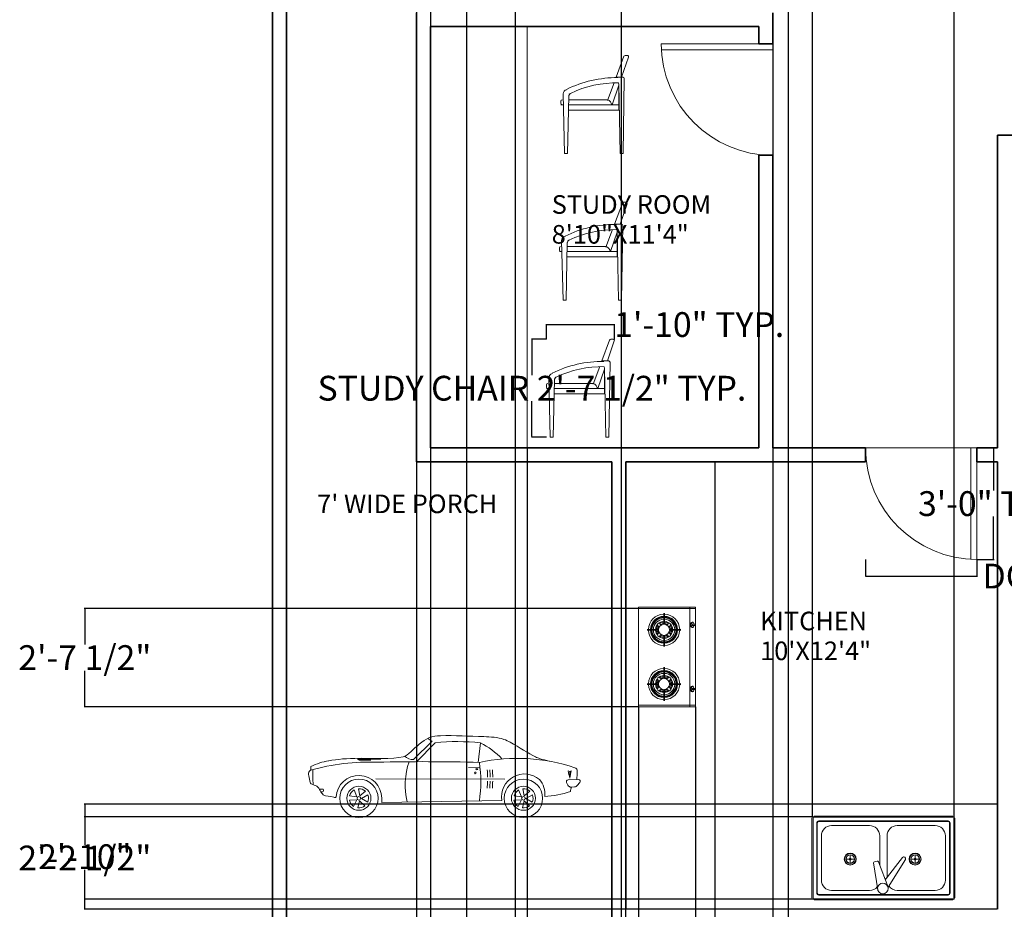
# Model space of a CAD drawing. Units: inches. Extents: x -438 to 102, y -60 to 1091.
# Tile 2 of 20: x -436 to -118, y 205 to 492. Entities that reach past the tile are written whole.
import ezdxf

# ---------------------------------------------------------------- set-up
doc = ezdxf.new("R2010")
doc.units = ezdxf.units.IN
doc.header["$MEASUREMENT"] = 0
for name, color, linetype, lineweight, true_color in [('A-ANNO-DIMS', 217, 'Continuous', 18, 0x93278f), ('A-DOOR', 30, 'Continuous', 18, 0xf26722), ('A-WALL', 2, 'Continuous', 35, 0xf1eb1f), ('C-PROP', 2, 'Continuous', 35, 0xf1eb1f)]:
    doc.layers.add(name, color=color, linetype=linetype, lineweight=lineweight, true_color=true_color)
for name, color, linetype, lineweight in [('A-AREA-IDEN', 4, 'Continuous', 18), ('A-EQPM', 9, 'Continuous', 15), ('A-FLOR-CASE', 7, 'Continuous', 18), ('A-FLOR-FIXT', 9, 'Continuous', 15), ('C-SITE-VEHI', 8, 'Continuous', 15), ('Furniture', 7, 'Continuous', 15)]:
    doc.layers.add(name, color=color, linetype=linetype, lineweight=lineweight)
doc.styles.get("Standard").update_dxf_attribs({"font": 'arial.ttf'})
doc.dimstyles.get("Standard").update_dxf_attribs({"dimtxt": 8, "dimasz": 0.18, "dimexe": 0.18, "dimexo": 0.0625, "dimgap": 0.09, "dimtad": 0, "dimtih": 1, "dimtoh": 1, "dimdec": 4, "dimzin": 0, "dimdsep": 46, "dimlunit": 3, "dimtxsty": 'Standard', "dimcen": 0.09, "dimadec": 0, "dimazin": 0, "dimtfac": 1, "dimtdec": 4, "dimtofl": 0, "dimtmove": 0, "dimatfit": 3, "dimfxl": 1, "dimtolj": 1, "dimtzin": 0, "dimarcsym": 0})

# ---------------------------------------------------------------- blocks, each defined once
blk = doc.blocks.new('*U3')
for p, q in [((72.93, 40.23), (85.8, 53.18)), ((75, 38.82), (88.08, 51.97)), ((119.39, 51.91), (117.92, 38.32)), ((50.13, 41.06), (34.31, 40.98)), ((43.26, 39.85), (35.15, 39.78)), ((35.3, 40.46), (50.13, 40.62)), ((111.09, 34.73), (118.48, 34.64)), ((46.65, 26.83), (136.29, 26.77)), ((179.3, 24.35), (180.25, 22.49)), ((180.37, 26.17), (187.51, 26.41)), ((182.62, 21.14), (184.91, 21.28)), ((186.68, 22.17), (188.51, 24.37)), ((7.45, 19.78), (9.74, 19.8)), ((9.76, 17.93), (8.53, 17.92)), ((10.37, 19.19), (10.38, 18.56)), ((50.87, 13.52), (50.91, 10.52))]:
    blk.add_line(p, q)
for points in [[(35.31, 39.93), (35.3, 40.27, 0.269532), (35.14, 40.54), (34.38, 40.96, 0.575383), (34.15, 40.83), (34.15, 40.49, 0.269532), (34.32, 40.22), (35.08, 39.79, 0.575383)], [(28.49, 15.1), (33.61, 14.4), (31.65, 19.18, 0.199906)], [(34.64, 20.05), (35.56, 14.97), (39.5, 18.31, 0.199906)], [(41.25, 15.74), (36.7, 13.3), (41.09, 10.58, 0.199906)], [(142.85, 15.1), (147.96, 14.4), (146.01, 19.18, 0.199906)], [(148.99, 20.05), (149.91, 14.97), (153.85, 18.31, 0.199906)], [(155.6, 15.74), (151.06, 13.3), (155.45, 10.58, 0.199906)], [(31.31, 7.72), (33.55, 12.37), (28.4, 11.99, 0.199906)], [(39.19, 8.12), (35.46, 11.69), (34.23, 6.67, 0.199906)], [(145.66, 7.72), (147.9, 12.37), (142.75, 11.99, 0.199906)], [(153.54, 8.12), (149.81, 11.69), (148.59, 6.67, 0.199906)]]:
    blk.add_lwpolyline(points, format="xyb", close=True)
for points in [[(181.58, 27.46), (181.53, 31.95), (180.48, 32.43)], [(181.58, 27.46), (181.53, 31.95), (182.57, 32.45)], [(50.91, 10.52), (134.38, 11.83)]]:
    blk.add_lwpolyline(points)
for centre, radius in [((115.89, 31.01), 0.619), ((34.98, 13.35), 13.35), ((34.98, 13.35), 8.35), ((149.33, 13.35), 13.35), ((149.33, 13.35), 8.35), ((34.98, 13.35), 1.25), ((149.33, 13.35), 1.25)]:
    blk.add_circle(centre, radius)
for centre, radius, start, end in [((114.6, 105.09), 59.37, 237.61027, 240.97846), ((103.45, -95), 147.78, 83.81633, 95.97054), ((95.51, 3.91), 53.61, 43.27479, 63.56652), ((73.29, 50.49), 10.26, 230.42401, 268.00854), ((145.17, -84.88), 125.99, 71.52833, 102.12419), ((42.18, -111.35), 149.91, 87.83928, 105.80965), ((20.53, -3.15), 43.06, 98.53035, 116.11198), ((80.1, -1364.13), 1402.96, 88.42296, 91.3179), ((118.31, 22.51), 51.16, 161.43071, 193.23633), ((25.66, 24.94), 94.01, 351.8279, 8.16738), ((184.3, 32.25), 2.49, 357.93203, 71.52833), ((79.16, 30.11), 76.3, 177.57734, 185.52052), ((34.98, 13.35), 15.9, 0.63732, 176.34123), ((45.64, 26.83), 78.76, 0.85201, 4.65562), ((47.43, 26.85), 78.76, 0.85201, 4.65562), ((49.23, 26.87), 78.76, 0.85201, 4.65562), ((150.1, 14.36), 15.92, 49.2263, 189.1528), ((216.26, 37.76), 36.17, 188.46832, 196.53145), ((146.68, 36.98), 36.17, 344.74319, 352.80633), ((116.55, 34.7), 70.29, 353.19423, 357.93203), ((45.64, 26.83), 78.76, 355.26443, 358.86328), ((47.43, 26.85), 78.76, 355.26443, 358.86328), ((49.23, 26.87), 78.76, 355.26443, 358.86328), ((149.4, 16.55), 14.84, 352.72855, 41.66131), ((180.41, 24.92), 1.25, 91.93898, 207.10902), ((182.47, 23.63), 2.49, 207.10902, 273.46767), ((114.25, 37.03), 70.29, 344.3985, 346.93849), ((184.76, 23.76), 2.49, 273.46767, 320.16835), ((187.55, 25.16), 1.25, 320.16835, 91.93898), ((9.75, 19.18), 0.623, 0.63732, 90.63732), ((9.76, 18.55), 0.623, 270.63732, 0.63732), ((162.47, 70.82), 56.18, 271.6865, 290.2774)]:
    blk.add_arc(centre, radius, start, end)
blk.add_ellipse((116.89, 33.59), major_axis=(-0.63, -0.007), ratio=0.610043)
for points, knots in [([(11.39, 38.92), (18.06, 40.19), (30.91, 42.01), (64.77, 40.11), (70.25, 44.91), (82.35, 56.38), (99.18, 57.3), (116.06, 56.35), (133.04, 55.87), (145.24, 49.87), (153.62, 43.8), (161.17, 40.68), (164.92, 39.73), (167.29, 39.15)], [18.629823, 18.629823, 18.629823, 18.629823, 19.527405, 20.700571, 21.107983, 21.608568, 21.92336, 23.151359, 23.716171, 23.908743, 24.77794, 24.943072, 25.187755, 25.187755, 25.187755, 25.187755]), ([(19.11, 14.36), (18.99, 14.21), (18.5, 13.81), (15.35, 15), (9.19, 13.94), (7.26, 22.22), (3.01, 22.66), (1.32, 23.61), (0.64, 26.92), (-0.96, 31.49), (1.54, 32.64), (1.5, 34.06), (1.49, 34.8), (1.49, 35.06), (1.52, 35.3), (1.58, 35.51)], [16.815853, 16.815853, 16.815853, 16.815853, 16.838212, 16.885395, 17.18439, 17.479846, 17.654423, 17.670693, 17.696923, 18.016358, 18.052739, 18.140805, 18.140805, 18.140805, 18.172382, 18.172382, 18.172382, 18.172382])]:
    blk.add_open_spline(points, degree=3, knots=knots)
blk = doc.blocks.new('CHAIR-STUDY')
for p, q in [((9.42, 15.56, -13.5), (6.9, 8.79, -13.5)), ((8.67, 8.79, -13.5), (10.91, 15.29, -13.5)), ((10.54, 15.81, -13.5), (9.79, 15.81, -13.5)), ((6.24, 7.02, -13.5), (4.1, 1.29, -13.5)), ((6.9, 8.79, -13.5), (7.01, 8.79, -13.5)), ((8.16, -15.81, -13.5), (7.76, 6.63, -13.5)), ((7.76, 6.63, -13.5), (7.76, -1.84, -13.5)), ((8.08, 8.79, -13.5), (9.14, 8.79, -13.5)), ((9.14, -15.81, -13.5), (9.54, 8.4, -13.5)), ((-9.76, -15.81, -13.5), (-10.23, 3.39, -13.5)), ((5.6, -0.06, -13.5), (7.76, 6.19, -13.5)), ((-10.94, 0.33, -13.5), (-10.94, 1.12, -13.5)), ((-8.77, -15.81, -13.5), (-8.38, 2.84, -13.5)), ((-8.38, 1.51, -13.5), (4.18, 1.51, -13.5)), ((-10.15, -0.06, -13.5), (-10.94, -0.06, -13.5)), ((-8.38, -0.06, -13.5), (7.76, -0.06, -13.5)), ((7.76, -1.84, -13.5), (-8.38, -1.84, -13.5)), ((7.76, -0.06, -13.5), (5.6, -0.06, -13.5)), ((-8.77, -15.81, -13.5), (-9.76, -15.81, -13.5)), ((9.14, -15.81, -13.5), (8.16, -15.81, -13.5))]:
    blk.add_line(p, q)
for centre, radius, start, end in [((9.79, 15.42, -13.5), 0.394, 90, 159.543), ((10.54, 15.42, -13.5), 0.394, 340.9062, 90), ((7.23, -28.38, -13.5), 37.06, 89.5909, 116.1955), ((7.15, -27.86, -13.5), 34.85, 89.1298, 115.4866), ((7.54, -30.56, -13.5), 39.36, 88.7797, 90.7752), ((7.37, 6.63, -13.5), 0.394, 0, 66.9425), ((9.14, 8.4, -13.5), 0.394, 0, 90), ((-8.76, 3.36, -13.5), 1.47, 106.2385, 178.6251), ((-9.11, 3.69, -13.5), 1.19, 84.4727, 90.6658), ((-7.33, 2.68, -13.5), 1.06, 104.0799, 187.3471), ((7.41, -29.45, -13.5), 36.44, 115.6772, 115.6838), ((-10.54, 1.12, -13.5), 0.394, 90, 180), ((-10.54, 0.33, -13.5), 0.394, 180, 270), ((3.59, -0.28, -13.5), 1.88, 6.4482, 71.4849)]:
    blk.add_arc(centre, radius, start, end)
blk = doc.blocks.new('DOOR-SWING-36')
for p, q in [((-36, 0), (0, 0)), ((-2, 0), (-2, -36)), ((0, 0), (0, -36))]:
    blk.add_line(p, q)
blk.add_arc((0, 0), 36, 180, 270)
blk = doc.blocks.new('*D16')
at = {"layer": 'A-ANNO-DIMS', "color": 0, "lineweight": -2, "transparency": 16777216}
for p, q in [((-265.73, 389.07), (-270.59, 389.07)), ((-270.41, 388.89), (-270.41, 377.48)), ((-270.41, 357.62), (-270.41, 369.03)), ((-265.73, 357.44), (-270.59, 357.44))]:
    blk.add_line(p, q, dxfattribs=at)
at = {"layer": 'A-ANNO-DIMS', "color": 0, "transparency": 16777216}
for points in [[(-270.44, 388.89), (-270.38, 388.89), (-270.41, 389.07)], [(-270.44, 357.62), (-270.38, 357.62), (-270.41, 357.44)]]:
    blk.add_solid(points, dxfattribs=at)
at = {"layer": 'Defpoints', "color": 0, "transparency": 16777216}
for p in [(-270.41, 389.07), (-265.67, 389.07), (-265.67, 357.44)]:
    blk.add_point(p, dxfattribs=at)
at = {"layer": 'A-ANNO-DIMS', "color": 0, "transparency": 16777216, "insert": (-270.41, 373.26), "char_height": 8, "attachment_point": 5}
blk.add_mtext('\\A1;STUDY CHAIR 2\'-7 1/2" TYP.', dxfattribs=at)
blk = doc.blocks.new('*D17')
at = {"layer": 'A-ANNO-DIMS', "color": 0, "lineweight": -2, "transparency": 16777216}
for p, q in [((-265.67, 389.13), (-265.67, 393.99)), ((-265.49, 393.81), (-243.96, 393.81)), ((-243.78, 389.13), (-243.78, 393.99)), ((-243.78, 393.81), (-243.6, 393.81))]:
    blk.add_line(p, q, dxfattribs=at)
at = {"layer": 'A-ANNO-DIMS', "color": 0, "transparency": 16777216}
for points in [[(-265.49, 393.84), (-265.49, 393.78), (-265.67, 393.81)], [(-243.96, 393.84), (-243.96, 393.78), (-243.78, 393.81)]]:
    blk.add_solid(points, dxfattribs=at)
at = {"layer": 'Defpoints', "color": 0, "transparency": 16777216}
for p in [(-243.78, 393.81), (-265.67, 389.07), (-243.78, 389.07)]:
    blk.add_point(p, dxfattribs=at)
at = {"layer": 'A-ANNO-DIMS', "color": 0, "transparency": 16777216, "insert": (-216.4, 393.81), "char_height": 8, "attachment_point": 5}
blk.add_mtext('\\A1;1\'-10" TYP.', dxfattribs=at)
blk = doc.blocks.new('*D20')
at = {"layer": 'A-ANNO-DIMS', "color": 0, "lineweight": -2, "transparency": 16777216}
for p, q in [((-162.74, 317.94), (-162.74, 312.42)), ((-126.74, 317.94), (-126.74, 312.42)), ((-162.56, 312.6), (-126.92, 312.6)), ((-126.74, 312.6), (-126.56, 312.6))]:
    blk.add_line(p, q, dxfattribs=at)
at = {"layer": 'A-ANNO-DIMS', "color": 0, "transparency": 16777216}
for points in [[(-162.56, 312.63), (-162.56, 312.57), (-162.74, 312.6)], [(-126.92, 312.63), (-126.92, 312.57), (-126.74, 312.6)]]:
    blk.add_solid(points, dxfattribs=at)
at = {"layer": 'Defpoints', "color": 0, "transparency": 16777216}
for p in [(-162.74, 318), (-126.74, 318), (-126.74, 312.6)]:
    blk.add_point(p, dxfattribs=at)
at = {"layer": 'A-ANNO-DIMS', "color": 0, "transparency": 16777216, "insert": (-83.97, 312.6), "char_height": 8, "attachment_point": 5}
blk.add_mtext('\\A1;DOOR 3\'-0" TYP.', dxfattribs=at)
blk = doc.blocks.new('*D21')
at = {"layer": 'A-ANNO-DIMS', "color": 0, "lineweight": -2, "transparency": 16777216}
for p, q in [((-126.67, 354), (-121.16, 354)), ((-121.34, 353.82), (-121.34, 340.18)), ((-121.34, 318.18), (-121.34, 331.82)), ((-126.67, 318), (-121.16, 318))]:
    blk.add_line(p, q, dxfattribs=at)
at = {"layer": 'A-ANNO-DIMS', "color": 0, "transparency": 16777216}
for points in [[(-121.37, 353.82), (-121.31, 353.82), (-121.34, 354)], [(-121.37, 318.18), (-121.31, 318.18), (-121.34, 318)]]:
    blk.add_solid(points, dxfattribs=at)
at = {"layer": 'Defpoints', "color": 0, "transparency": 16777216}
for p in [(-126.74, 354), (-121.34, 354), (-126.74, 318)]:
    blk.add_point(p, dxfattribs=at)
at = {"layer": 'A-ANNO-DIMS', "color": 0, "transparency": 16777216, "insert": (-121.34, 336), "char_height": 8, "attachment_point": 5}
blk.add_mtext('\\A1;3\'-0" TYP.', dxfattribs=at)
blk = doc.blocks.new('*D28')
at = {"layer": 'A-ANNO-DIMS', "color": 0, "lineweight": -2, "transparency": 16777216}
for p, q in [((-303.15, 353.94), (-303.15, -48.58)), ((-271.99, 353.94), (-271.99, -48.58)), ((-302.97, -48.4), (-298.36, -48.4)), ((-272.17, -48.4), (-276.78, -48.4))]:
    blk.add_line(p, q, dxfattribs=at)
at = {"layer": 'A-ANNO-DIMS', "color": 0, "transparency": 16777216}
for points in [[(-302.97, -48.37), (-302.97, -48.43), (-303.15, -48.4)], [(-272.17, -48.37), (-272.17, -48.43), (-271.99, -48.4)]]:
    blk.add_solid(points, dxfattribs=at)
at = {"layer": 'Defpoints', "color": 0, "transparency": 16777216}
for p in [(-303.15, 354), (-271.99, 354), (-271.99, -48.4)]:
    blk.add_point(p, dxfattribs=at)
at = {"layer": 'A-ANNO-DIMS', "color": 0, "transparency": 16777216, "insert": (-287.57, -48.4), "char_height": 8, "attachment_point": 5}
blk.add_mtext('\\A1;2\'-7"', dxfattribs=at)
blk = doc.blocks.new('*D29')
at = {"layer": 'A-ANNO-DIMS', "color": 0, "lineweight": -2, "transparency": 16777216}
for p, q in [((-303.15, 494.44), (-303.15, -48.58)), ((-192.65, 494.44), (-192.65, -48.58)), ((-302.97, -48.4), (-267.94, -48.4)), ((-192.83, -48.4), (-227.85, -48.4))]:
    blk.add_line(p, q, dxfattribs=at)
at = {"layer": 'A-ANNO-DIMS', "color": 0, "transparency": 16777216}
for points in [[(-302.97, -48.37), (-302.97, -48.43), (-303.15, -48.4)], [(-192.83, -48.37), (-192.83, -48.43), (-192.65, -48.4)]]:
    blk.add_solid(points, dxfattribs=at)
at = {"layer": 'Defpoints', "color": 0, "transparency": 16777216}
for p in [(-303.15, 494.5), (-192.65, 494.5), (-192.65, -48.4)]:
    blk.add_point(p, dxfattribs=at)
at = {"layer": 'A-ANNO-DIMS', "color": 0, "transparency": 16777216, "insert": (-247.9, -48.4), "char_height": 8, "attachment_point": 5}
blk.add_mtext('\\A1;9\'-2 1/2"', dxfattribs=at)
blk = doc.blocks.new('*D32')
at = {"layer": 'A-ANNO-DIMS', "color": 0, "lineweight": -2, "transparency": 16777216}
for p, q in [((-303.15, 584.44), (-303.15, -48.58)), ((-307.65, 579.94), (-307.65, -48.58)), ((-307.47, -48.4), (-303.33, -48.4)), ((-303.15, -48.4), (-302.97, -48.4))]:
    blk.add_line(p, q, dxfattribs=at)
at = {"layer": 'A-ANNO-DIMS', "color": 0, "transparency": 16777216}
for points in [[(-307.47, -48.37), (-307.47, -48.43), (-307.65, -48.4)], [(-303.33, -48.37), (-303.33, -48.43), (-303.15, -48.4)]]:
    blk.add_solid(points, dxfattribs=at)
at = {"layer": 'Defpoints', "color": 0, "transparency": 16777216}
for p in [(-303.15, 584.5), (-307.65, 580), (-303.15, -48.4)]:
    blk.add_point(p, dxfattribs=at)
at = {"layer": 'A-ANNO-DIMS', "color": 0, "transparency": 16777216, "insert": (-282.92, -48.4), "char_height": 8, "attachment_point": 5}
blk.add_mtext('\\A1;0\'-4 1/2"', dxfattribs=at)
blk = doc.blocks.new('*D33')
at = {"layer": 'A-ANNO-DIMS', "color": 0, "lineweight": -2, "transparency": 16777216}
for p, q in [((-240.15, 349.44), (-240.15, -48.58)), ((-211.32, 349.44), (-211.32, -48.58)), ((-239.97, -48.4), (-236.52, -48.4)), ((-211.5, -48.4), (-214.94, -48.4))]:
    blk.add_line(p, q, dxfattribs=at)
at = {"layer": 'A-ANNO-DIMS', "color": 0, "transparency": 16777216}
for points in [[(-239.97, -48.37), (-239.97, -48.43), (-240.15, -48.4)], [(-211.5, -48.37), (-211.5, -48.43), (-211.32, -48.4)]]:
    blk.add_solid(points, dxfattribs=at)
at = {"layer": 'Defpoints', "color": 0, "transparency": 16777216}
for p in [(-240.15, 349.5), (-211.32, 349.5), (-211.32, -48.4)]:
    blk.add_point(p, dxfattribs=at)
at = {"layer": 'A-ANNO-DIMS', "color": 0, "transparency": 16777216, "insert": (-225.73, -48.4), "char_height": 8, "attachment_point": 5}
blk.add_mtext('\\A1;2\'-5"', dxfattribs=at)
blk = doc.blocks.new('*D34')
at = {"layer": 'A-ANNO-DIMS', "color": 0, "lineweight": -2, "transparency": 16777216}
for p, q in [((-120.21, 238.94), (-414.94, 238.94)), ((-414.76, 238.76), (-414.76, 226.14)), ((-414.76, 205.18), (-414.76, 217.79)), ((-120.21, 205), (-414.94, 205))]:
    blk.add_line(p, q, dxfattribs=at)
at = {"layer": 'A-ANNO-DIMS', "color": 0, "transparency": 16777216}
for points in [[(-414.79, 238.76), (-414.73, 238.76), (-414.76, 238.94)], [(-414.79, 205.18), (-414.73, 205.18), (-414.76, 205)]]:
    blk.add_solid(points, dxfattribs=at)
at = {"layer": 'Defpoints', "color": 0, "transparency": 16777216}
for p in [(-120.15, 238.94), (-414.76, 205), (-120.15, 205)]:
    blk.add_point(p, dxfattribs=at)
at = {"layer": 'A-ANNO-DIMS', "color": 0, "transparency": 16777216, "insert": (-414.76, 221.97), "char_height": 8, "attachment_point": 5}
blk.add_mtext('\\A1;2\'-10"', dxfattribs=at)
blk = doc.blocks.new('*D37')
at = {"layer": 'A-ANNO-DIMS', "color": 0, "lineweight": -2, "transparency": 16777216}
for p, q in [((-179.8, 234.94), (-179.8, 1079.58)), ((-179.62, 1079.4), (-176.98, 1079.4)), ((-134.26, 1079.4), (-136.9, 1079.4)), ((-134.08, 234.94), (-134.08, 1079.58))]:
    blk.add_line(p, q, dxfattribs=at)
at = {"layer": 'A-ANNO-DIMS', "color": 0, "transparency": 16777216}
for points in [[(-179.62, 1079.43), (-179.62, 1079.37), (-179.8, 1079.4)], [(-134.26, 1079.43), (-134.26, 1079.37), (-134.08, 1079.4)]]:
    blk.add_solid(points, dxfattribs=at)
at = {"layer": 'Defpoints', "color": 0, "transparency": 16777216}
for p in [(-134.08, 1079.4), (-179.8, 234.88), (-134.08, 234.88)]:
    blk.add_point(p, dxfattribs=at)
at = {"layer": 'A-ANNO-DIMS', "color": 0, "transparency": 16777216, "insert": (-156.94, 1079.4), "char_height": 8, "attachment_point": 5}
blk.add_mtext('\\A1;3\'-9 1/2"', dxfattribs=at)
blk = doc.blocks.new('*D38')
at = {"layer": 'A-ANNO-DIMS', "color": 0, "lineweight": -2, "transparency": 16777216}
for p, q in [((-179.86, 234.88), (-414.94, 234.88)), ((-414.76, 234.7), (-414.76, 225.8)), ((-414.76, 208.44), (-414.76, 217.34)), ((-179.86, 208.26), (-414.94, 208.26))]:
    blk.add_line(p, q, dxfattribs=at)
at = {"layer": 'A-ANNO-DIMS', "color": 0, "transparency": 16777216}
for points in [[(-414.79, 234.7), (-414.73, 234.7), (-414.76, 234.88)], [(-414.79, 208.44), (-414.73, 208.44), (-414.76, 208.26)]]:
    blk.add_solid(points, dxfattribs=at)
at = {"layer": 'Defpoints', "color": 0, "transparency": 16777216}
for p in [(-414.76, 234.88), (-179.8, 234.88), (-179.8, 208.26)]:
    blk.add_point(p, dxfattribs=at)
at = {"layer": 'A-ANNO-DIMS', "color": 0, "transparency": 16777216, "insert": (-414.76, 221.57), "char_height": 8, "attachment_point": 5}
blk.add_mtext('\\A1;2\'-2 1/2"', dxfattribs=at)
blk = doc.blocks.new('*D39')
at = {"layer": 'A-ANNO-DIMS', "color": 0, "lineweight": -2, "transparency": 16777216}
for p, q in [((-236.04, 302.11), (-414.94, 302.11)), ((-414.76, 301.93), (-414.76, 290.49)), ((-414.76, 270.6), (-414.76, 282.04)), ((-236.04, 270.42), (-414.94, 270.42))]:
    blk.add_line(p, q, dxfattribs=at)
at = {"layer": 'A-ANNO-DIMS', "color": 0, "transparency": 16777216}
for points in [[(-414.79, 301.93), (-414.73, 301.93), (-414.76, 302.11)], [(-414.79, 270.6), (-414.73, 270.6), (-414.76, 270.42)]]:
    blk.add_solid(points, dxfattribs=at)
at = {"layer": 'Defpoints', "color": 0, "transparency": 16777216}
for p in [(-235.98, 302.11), (-414.76, 270.42), (-235.98, 270.42)]:
    blk.add_point(p, dxfattribs=at)
at = {"layer": 'A-ANNO-DIMS', "color": 0, "transparency": 16777216, "insert": (-414.76, 286.27), "char_height": 8, "attachment_point": 5}
blk.add_mtext('\\A1;2\'-7 1/2"', dxfattribs=at)
blk = doc.blocks.new('*D40')
at = {"layer": 'A-ANNO-DIMS', "color": 0, "lineweight": -2, "transparency": 16777216}
for p, q in [((-235.98, 270.35), (-235.98, -48.58)), ((-217.6, 270.35), (-217.6, -48.58)), ((-235.8, -48.4), (-217.78, -48.4)), ((-217.6, -48.4), (-217.42, -48.4))]:
    blk.add_line(p, q, dxfattribs=at)
at = {"layer": 'A-ANNO-DIMS', "color": 0, "transparency": 16777216}
for points in [[(-235.8, -48.37), (-235.8, -48.43), (-235.98, -48.4)], [(-217.78, -48.37), (-217.78, -48.43), (-217.6, -48.4)]]:
    blk.add_solid(points, dxfattribs=at)
at = {"layer": 'Defpoints', "color": 0, "transparency": 16777216}
for p in [(-235.98, 270.42), (-217.6, 270.42), (-217.6, -48.4)]:
    blk.add_point(p, dxfattribs=at)
at = {"layer": 'A-ANNO-DIMS', "color": 0, "transparency": 16777216, "insert": (-197.75, -48.4), "char_height": 8, "attachment_point": 5}
blk.add_mtext('\\A1;1\'-6 1/2"', dxfattribs=at)
blk = doc.blocks.new('*D51')
at = {"layer": 'A-ANNO-DIMS', "color": 0, "lineweight": -2, "transparency": 16777216}
for p, q in [((-291.54, 847), (-291.54, -48.58)), ((-275.79, 847), (-275.79, -48.58)), ((-291.36, -48.4), (-275.97, -48.4)), ((-275.79, -48.4), (-275.61, -48.4))]:
    blk.add_line(p, q, dxfattribs=at)
at = {"layer": 'A-ANNO-DIMS', "color": 0, "transparency": 16777216}
for points in [[(-291.36, -48.37), (-291.36, -48.43), (-291.54, -48.4)], [(-275.97, -48.37), (-275.97, -48.43), (-275.79, -48.4)]]:
    blk.add_solid(points, dxfattribs=at)
at = {"layer": 'Defpoints', "color": 0, "transparency": 16777216}
for p in [(-291.54, 847.06), (-275.79, 847.06), (-275.79, -48.4)]:
    blk.add_point(p, dxfattribs=at)
at = {"layer": 'A-ANNO-DIMS', "color": 0, "transparency": 16777216, "insert": (-255.95, -48.4), "char_height": 8, "attachment_point": 5}
blk.add_mtext('\\A1;1\'-3 1/2"', dxfattribs=at)
blk = doc.blocks.new('*D55')
at = {"layer": 'A-ANNO-DIMS', "color": 0, "lineweight": -2, "transparency": 16777216}
for p, q in [((-241.57, 808.32), (-241.57, -48.58)), ((-187.65, 801.94), (-187.65, -48.58)), ((-241.39, -48.4), (-225.49, -48.4)), ((-187.83, -48.4), (-203.72, -48.4))]:
    blk.add_line(p, q, dxfattribs=at)
at = {"layer": 'A-ANNO-DIMS', "color": 0, "transparency": 16777216}
for points in [[(-241.39, -48.37), (-241.39, -48.43), (-241.57, -48.4)], [(-187.83, -48.37), (-187.83, -48.43), (-187.65, -48.4)]]:
    blk.add_solid(points, dxfattribs=at)
at = {"layer": 'Defpoints', "color": 0, "transparency": 16777216}
for p in [(-241.57, 808.38), (-187.65, 802), (-187.65, -48.4)]:
    blk.add_point(p, dxfattribs=at)
at = {"layer": 'A-ANNO-DIMS', "color": 0, "transparency": 16777216, "insert": (-214.61, -48.4), "char_height": 8, "attachment_point": 5}
blk.add_mtext('\\A1;4\'-6"', dxfattribs=at)

msp = doc.modelspace()

# ---------------------------------------------------------------- linework, layer by layer
at = {"layer": 'A-EQPM'}
for p, q in [((-217.59887, 302.57397), (-235.97515, 302.57397)), ((-235.97515, 302.57397), (-235.97515, 270.41548)), ((-217.59887, 302.11457), (-235.97515, 302.11457)), ((-219.4365, 270.41548), (-219.4365, 302.57397)), ((-217.59887, 270.41548), (-217.59887, 302.57397)), ((-227.87388, 297.31181), (-227.87388, 300.65588)), ((-227.64418, 297.31181), (-227.64418, 300.65588)), ((-229.96313, 296.28231), (-230.20308, 296.52226)), ((-229.50915, 296.34809), (-230.00572, 296.84466)), ((-228.85945, 296.99779), (-229.35602, 297.49436)), ((-228.79367, 297.45177), (-229.03362, 297.69172)), ((-226.48444, 297.69172), (-226.72439, 297.45177)), ((-226.16204, 297.49436), (-226.65861, 296.99779)), ((-225.51234, 296.84466), (-226.00891, 296.34809)), ((-225.31498, 296.52226), (-225.55493, 296.28231)), ((-218.56749, 297.05179), (-218.82492, 297.05179)), ((-218.56749, 296.64296), (-218.8194, 296.64296)), ((-218.56105, 297.76543), (-218.72604, 297.76543)), ((-218.56105, 295.95175), (-218.72604, 295.95175)), ((-218.65937, 296.95991), (-218.65937, 296.73484)), ((-217.7926, 297.05179), (-218.56749, 297.05179)), ((-218.56749, 296.64296), (-217.7926, 296.64296)), ((-217.70072, 296.73484), (-217.70072, 296.95991)), ((-229.82317, 295.36252), (-233.22156, 295.36252)), ((-229.82317, 295.13282), (-233.22156, 295.13282)), ((-229.96313, 294.21303), (-230.20308, 293.97308)), ((-229.50915, 294.14725), (-230.00572, 293.65068)), ((-228.85945, 293.49755), (-229.35602, 293.00098)), ((-228.79367, 293.04357), (-229.03362, 292.80362)), ((-227.87388, 293.18353), (-227.87388, 289.80447)), ((-227.64418, 293.18353), (-227.64418, 289.80447)), ((-226.48444, 292.80362), (-226.72439, 293.04357)), ((-226.16204, 293.00098), (-226.65861, 293.49755)), ((-225.51234, 293.65068), (-226.00891, 294.14725)), ((-225.69489, 295.36252), (-222.38832, 295.36252)), ((-225.69489, 295.13282), (-222.38832, 295.13282)), ((-225.31498, 293.97308), (-225.55493, 294.21303)), ((-227.87388, 279.80593), (-227.87388, 283.18499)), ((-227.64418, 279.80593), (-227.64418, 283.18499)), ((-228.85945, 279.49191), (-229.35602, 279.98847)), ((-228.79367, 279.94589), (-229.03362, 280.18584)), ((-226.48444, 280.18584), (-226.72439, 279.94589)), ((-226.16204, 279.98847), (-226.65861, 279.49191)), ((-229.82317, 277.85664), (-233.22156, 277.85664)), ((-229.82317, 277.62694), (-233.22156, 277.62694)), ((-229.96313, 278.77643), (-230.20308, 279.01638)), ((-229.96313, 276.70715), (-230.20308, 276.46719)), ((-229.50915, 278.84221), (-230.00572, 279.33877)), ((-229.50915, 276.64136), (-230.00572, 276.1448)), ((-225.51234, 279.33877), (-226.00891, 278.84221)), ((-225.51234, 276.1448), (-226.00891, 276.64136)), ((-225.69489, 277.85664), (-222.38832, 277.85664)), ((-225.69489, 277.62694), (-222.38832, 277.62694)), ((-225.31498, 279.01638), (-225.55493, 278.77643)), ((-225.31498, 276.46719), (-225.55493, 276.70715)), ((-218.56105, 277.03771), (-218.72604, 277.03771)), ((-228.85945, 275.99166), (-229.35602, 275.4951)), ((-228.79367, 275.53769), (-229.03362, 275.29774)), ((-227.87388, 275.67765), (-227.87388, 272.33357)), ((-227.64418, 275.67765), (-227.64418, 272.33357)), ((-226.48444, 275.29774), (-226.72439, 275.53769)), ((-226.16204, 275.4951), (-226.65861, 275.99166)), ((-218.56749, 275.93767), (-218.82492, 275.93767)), ((-218.56749, 276.34649), (-218.8194, 276.34649)), ((-218.56105, 275.22403), (-218.72604, 275.22403)), ((-218.65937, 276.02955), (-218.65937, 276.25461)), ((-218.56749, 276.34649), (-217.7926, 276.34649)), ((-217.7926, 275.93767), (-218.56749, 275.93767)), ((-217.70072, 276.25461), (-217.70072, 276.02955)), ((-235.97515, 270.87489), (-217.59887, 270.87489)), ((-235.97515, 270.41548), (-217.59887, 270.41548))]:
    msp.add_line(p, q, dxfattribs=at)
for centre, radius in [((-227.75903, 295.24767), 1.79169), ((-224.78276, 297.48032), 0.16439), ((-224.513, 297.06379), 0.16439), ((-227.75903, 277.74179), 1.79169), ((-224.78276, 275.50913), 0.16439), ((-224.513, 275.92567), 0.16439)]:
    msp.add_circle(centre, radius, dxfattribs=at)
for centre, radius, start, end in [((-227.75903, 295.24767), 5.05348, 91.3022889, 178.6977111), ((-227.75903, 295.24767), 4.36437, 91.5917542, 178.4082458), ((-227.75903, 295.24767), 4.13466, 91.5917542, 178.4082458), ((-227.75903, 295.24767), 3.90496, 91.685413, 178.314587), ((-227.75903, 295.24767), 5.05348, 1.3022889, 88.6977111), ((-227.75903, 295.24767), 4.13466, 1.5917542, 88.4082458), ((-227.75903, 295.24767), 3.90496, 1.685413, 88.314587), ((-227.75903, 295.24767), 4.36437, 1.5917542, 88.4082458), ((-227.75903, 295.24767), 3.44555, 91.9102132, 178.0897868), ((-227.75903, 295.24767), 2.75644, 92.3880155, 177.6119845), ((-227.75903, 295.24767), 2.43486, 154.853885, 177.2963657), ((-227.75903, 295.24767), 2.06733, 147.8395884, 176.8152615), ((-227.75903, 295.24767), 2.06733, 93.1847385, 122.1604116), ((-227.75903, 295.24767), 2.43486, 92.7036343, 115.146115), ((-227.75903, 297.32537), 0.11565, 186.7353744, 353.2646256), ((-227.75903, 295.24767), 3.44555, 1.9102132, 88.0897868), ((-227.75903, 295.24767), 2.75644, 2.3880155, 87.6119845), ((-227.75903, 295.24767), 2.43486, 64.853885, 87.2963657), ((-227.75903, 295.24767), 2.06733, 57.8395884, 86.8152615), ((-227.75903, 295.24767), 2.06733, 3.1847385, 32.1604116), ((-227.75903, 295.24767), 2.43486, 2.7036343, 25.146115), ((-218.82492, 297.14367), 0.09188, 166.6924973, 270), ((-217.61965, 296.85859), 1.33041, 138.6513888, 166.6924973), ((-218.8194, 296.55108), 0.09188, 90, 194.3759834), ((-217.61965, 296.85859), 1.33041, 194.3759834, 219.6110848), ((-218.56749, 296.95991), 0.09188, 90, 180), ((-218.56749, 296.73484), 0.09188, 180, 270), ((-218.53961, 296.07115), 0.12131, 210.0749159, 302.1858261), ((-218.54942, 297.67681), 0.09188, 75.3271166, 138.6513888), ((-217.7926, 296.95991), 0.09188, 0, 90), ((-217.7926, 296.73484), 0.09188, 270, 0), ((-227.75903, 295.24767), 5.05348, 181.3022889, 268.6977111), ((-227.75903, 295.24767), 4.36437, 181.5917542, 268.4082458), ((-227.75903, 295.24767), 4.13466, 181.5917542, 268.4082458), ((-227.75903, 295.24767), 3.90496, 181.685413, 268.314587), ((-227.75903, 295.24767), 3.44555, 181.9102132, 268.0897868), ((-227.75903, 295.24767), 2.75644, 182.3880155, 267.6119845), ((-227.75903, 295.24767), 2.43486, 182.7036343, 205.146115), ((-229.86623, 295.24767), 0.12266, 290.550693, 69.449307), ((-227.75903, 295.24767), 2.06733, 183.1847385, 212.1604116), ((-227.75903, 295.24767), 2.06733, 237.8395884, 266.8152615), ((-227.75903, 295.24767), 2.43486, 244.853885, 267.2963657), ((-227.75903, 293.13762), 0.12369, 21.7885229, 158.2114771), ((-227.75903, 295.24767), 2.75644, 272.3880155, 357.6119845), ((-227.75903, 295.24767), 5.05348, 271.3022889, 358.6977111), ((-227.75903, 295.24767), 3.90496, 271.685413, 358.314587), ((-227.75903, 295.24767), 3.44555, 271.9102132, 358.0897868), ((-227.75903, 295.24767), 4.13466, 271.5917542, 358.4082458), ((-227.75903, 295.24767), 2.06733, 273.1847385, 302.1604116), ((-227.75903, 295.24767), 2.43486, 272.7036343, 295.146115), ((-227.75903, 295.24767), 4.36437, 271.5917542, 358.4082458), ((-227.75903, 295.24767), 2.06733, 327.8395884, 356.8152615), ((-225.6559, 295.24767), 0.12129, 108.751046, 251.248954), ((-227.75903, 295.24767), 2.43486, 334.853885, 357.2963657), ((-227.75903, 277.74179), 5.05348, 91.3022889, 178.6977111), ((-227.75903, 277.74179), 4.36437, 91.5917542, 178.4082458), ((-227.75903, 277.74179), 4.13466, 91.5917542, 178.4082458), ((-227.75903, 277.74179), 3.90496, 91.685413, 178.314587), ((-227.75903, 277.74179), 3.44555, 91.9102132, 178.0897868), ((-227.75903, 277.74179), 2.75644, 92.3880155, 177.6119845), ((-227.75903, 277.74179), 2.06733, 93.1847385, 122.1604116), ((-227.75903, 277.74179), 2.43486, 92.7036343, 115.146115), ((-227.75903, 279.85184), 0.12369, 201.7885229, 338.2114771), ((-227.75903, 277.74179), 5.05348, 1.3022889, 88.6977111), ((-227.75903, 277.74179), 4.13466, 1.5917542, 88.4082458), ((-227.75903, 277.74179), 3.90496, 1.685413, 88.314587), ((-227.75903, 277.74179), 3.44555, 1.9102132, 88.0897868), ((-227.75903, 277.74179), 2.75644, 2.3880155, 87.6119845), ((-227.75903, 277.74179), 2.43486, 64.853885, 87.2963657), ((-227.75903, 277.74179), 2.06733, 57.8395884, 86.8152615), ((-227.75903, 277.74179), 4.36437, 1.5917542, 88.4082458), ((-227.75903, 277.74179), 5.05348, 181.3022889, 268.6977111), ((-227.75903, 277.74179), 4.36437, 181.5917542, 268.4082458), ((-227.75903, 277.74179), 4.13466, 181.5917542, 268.4082458), ((-227.75903, 277.74179), 3.90496, 181.685413, 268.314587), ((-227.75903, 277.74179), 3.44555, 181.9102132, 268.0897868), ((-227.75903, 277.74179), 2.75644, 182.3880155, 267.6119845), ((-227.75903, 277.74179), 2.43486, 154.853885, 177.2963657), ((-227.75903, 277.74179), 2.43486, 182.7036343, 205.146115), ((-227.75903, 277.74179), 2.06733, 147.8395884, 176.8152615), ((-229.86623, 277.74179), 0.12266, 290.550693, 69.449307), ((-227.75903, 277.74179), 2.06733, 183.1847385, 212.1604116), ((-227.75903, 277.74179), 2.75644, 272.3880155, 357.6119845), ((-227.75903, 277.74179), 5.05348, 271.3022889, 358.6977111), ((-227.75903, 277.74179), 3.44555, 271.9102132, 358.0897868), ((-227.75903, 277.74179), 3.90496, 271.685413, 358.314587), ((-227.75903, 277.74179), 4.13466, 271.5917542, 358.4082458), ((-227.75903, 277.74179), 4.36437, 271.5917542, 358.4082458), ((-227.75903, 277.74179), 2.06733, 3.1847385, 32.1604116), ((-227.75903, 277.74179), 2.06733, 327.8395884, 356.8152615), ((-225.6559, 277.74179), 0.12129, 108.751046, 251.248954), ((-227.75903, 277.74179), 2.43486, 2.7036343, 25.146115), ((-227.75903, 277.74179), 2.43486, 334.853885, 357.2963657), ((-217.61965, 276.13087), 1.33041, 140.3889152, 165.6240166), ((-218.53961, 276.91831), 0.12131, 57.8141739, 149.9250841), ((-227.75903, 277.74179), 2.06733, 237.8395884, 266.8152615), ((-227.75903, 277.74179), 2.43486, 244.853885, 267.2963657), ((-227.75903, 275.66408), 0.11565, 6.7353744, 173.2646256), ((-227.75903, 277.74179), 2.06733, 273.1847385, 302.1604116), ((-227.75903, 277.74179), 2.43486, 272.7036343, 295.146115), ((-218.82492, 275.84579), 0.09188, 90, 193.3075027), ((-217.61965, 276.13087), 1.33041, 193.3075027, 221.3486112), ((-218.8194, 276.43838), 0.09188, 165.6240166, 270), ((-218.56749, 276.25461), 0.09188, 90, 180), ((-218.56749, 276.02955), 0.09188, 180, 270), ((-218.54942, 275.31265), 0.09188, 221.3486112, 284.6728834), ((-217.7926, 276.25461), 0.09188, 0, 90), ((-217.7926, 276.02955), 0.09188, 270, 0)]:
    msp.add_arc(centre, radius, start, end, dxfattribs=at)
at = {"layer": 'A-EQPM', "extrusion": (0, 0, -1)}
for start_param, end_param in [(3.311146783, 6.113631178), (0.167831346, 1.359229349), (1.807363774, 2.885845936)]:
    msp.add_ellipse((-218.62559, 296.85859), major_axis=(0, 0.92003), ratio=0.64705753, start_param=start_param, end_param=end_param, dxfattribs=at)
at = {"layer": 'A-EQPM'}
for start_param, end_param in [(3.311146783, 6.113631178), (1.807363774, 2.885845936), (0.167831346, 1.359229349)]:
    msp.add_ellipse((-218.62559, 276.13087), major_axis=(0, -0.92003), ratio=0.64705753, start_param=start_param, end_param=end_param, dxfattribs=at)
at = {"layer": 'A-FLOR-CASE'}
for p, q in [((-271.98824, 353.99939), (-271.98824, 489.99939)), ((-211.31973, 349.49939), (-211.31973, 238.93709)), ((-211.31973, 238.93709), (-120.14649, 238.93709))]:
    msp.add_line(p, q, dxfattribs=at)
at = {"layer": 'A-FLOR-FIXT'}
for p, q in [((-179.98875, 234.41276), (-179.98875, 208.72726)), ((-179.65945, 234.41276), (-179.65945, 208.72726)), ((-134.54519, 235.07136), (-179.33015, 235.07136)), ((-134.54519, 234.74206), (-179.33015, 234.74206)), ((-178.47397, 232.89797), (-178.47397, 210.24205)), ((-178.27639, 232.89797), (-178.27639, 210.24205)), ((-136.05997, 233.55658), (-177.81536, 233.55658)), ((-136.05997, 233.359), (-177.81536, 233.359)), ((-135.59895, 210.24205), (-135.59895, 232.89797)), ((-135.40137, 210.24205), (-135.40137, 232.89797)), ((-134.21588, 208.72726), (-134.21588, 234.41276)), ((-133.88658, 208.72726), (-133.88658, 234.41276)), ((-161.41616, 232.04179), (-173.66617, 232.04179)), ((-140.20917, 232.04179), (-152.45917, 232.04179)), ((-176.95918, 228.74878), (-176.95918, 214.39125)), ((-158.12315, 219.27764), (-158.12315, 228.74878)), ((-155.75218, 228.74878), (-155.75218, 215.20665)), ((-136.91615, 214.39125), (-136.91615, 228.74878)), ((-167.63944, 221.55712), (-167.63944, 222.54494)), ((-146.69926, 221.55712), (-146.69926, 222.54494)), ((-167.98048, 221.21608), (-168.9683, 221.21608)), ((-167.63944, 220.87504), (-167.63944, 219.88722)), ((-167.2984, 221.21608), (-166.31058, 221.21608)), ((-160.09137, 219.98181), (-158.76237, 211.29523)), ((-158.92904, 220.58514), (-159.84733, 220.35068)), ((-155.43599, 212.14739), (-158.53943, 220.38221)), ((-156.31387, 214.4768), (-150.73842, 221.72152)), ((-155.43599, 212.14739), (-149.83292, 221.08989)), ((-150.00844, 221.82443), (-149.96697, 221.79389)), ((-147.0403, 221.21608), (-148.02812, 221.21608)), ((-146.69926, 220.87504), (-146.69926, 219.88722)), ((-146.35822, 221.21608), (-145.3704, 221.21608)), ((-173.66617, 211.09823), (-161.41616, 211.09823)), ((-152.45917, 211.09823), (-140.20917, 211.09823)), ((-179.33015, 208.39796), (-134.54519, 208.39796)), ((-179.33015, 208.06866), (-134.54519, 208.06866)), ((-177.81536, 209.78103), (-136.05997, 209.78103)), ((-177.81536, 209.58345), (-136.05997, 209.58345))]:
    msp.add_line(p, q, dxfattribs=at)
for centre, radius in [((-167.63944, 221.21608), 1.94392), ((-167.63944, 221.21608), 1.83901), ((-167.63944, 221.21608), 1.38852), ((-167.63944, 221.21608), 1.32886), ((-146.69926, 221.21608), 1.94392), ((-146.69926, 221.21608), 1.83901), ((-146.69926, 221.21608), 1.38852), ((-146.69926, 221.21608), 1.32886), ((-167.63944, 221.21608), 0.34104), ((-167.63944, 221.21608), 0.16025), ((-146.69926, 221.21608), 0.34104), ((-146.69926, 221.21608), 0.16025), ((-157.09918, 211.72131), 1.7169)]:
    msp.add_circle(centre, radius, dxfattribs=at)
for centre, radius, start, end in [((-179.33015, 234.41276), 0.6586, 90, 180), ((-179.33015, 234.41276), 0.3293, 90, 180), ((-177.81536, 232.89797), 0.6586, 90, 180), ((-177.81536, 232.89797), 0.46102, 90, 180), ((-136.05997, 232.89797), 0.6586, 0, 90), ((-136.05997, 232.89797), 0.46102, 0, 90), ((-134.54519, 234.41276), 0.6586, 0, 90), ((-134.54519, 234.41276), 0.3293, 0, 90), ((-173.66617, 228.74878), 3.29301, 90, 180), ((-161.41616, 228.74878), 3.29301, 0, 90), ((-152.45917, 228.74878), 3.29301, 90, 180), ((-140.20917, 228.74878), 3.29301, 0, 90), ((-159.76586, 220.03161), 0.3293, 104.3233276, 188.6985351), ((-158.84758, 220.26608), 0.3293, 20.6498216, 104.3233276), ((-150.32087, 221.40018), 0.52688, 53.6309311, 142.4185447), ((-150.2794, 221.36964), 0.52688, 327.9301426, 53.6309311), ((-173.66617, 214.39125), 3.29301, 180, 270), ((-140.20917, 214.39125), 3.29301, 270, 0), ((-177.81536, 210.24205), 0.6586, 180, 270), ((-177.81536, 210.24205), 0.46102, 180, 270), ((-161.41616, 214.39125), 3.29301, 270, 319.5750097), ((-152.45917, 214.39125), 3.29301, 214.0864438, 270), ((-136.05997, 210.24205), 0.46102, 270, 0), ((-136.05997, 210.24205), 0.6586, 270, 0), ((-179.33015, 208.72726), 0.6586, 180, 270), ((-179.33015, 208.72726), 0.3293, 180, 270), ((-134.54519, 208.72726), 0.3293, 270, 0), ((-134.54519, 208.72726), 0.6586, 270, 0)]:
    msp.add_arc(centre, radius, start, end, dxfattribs=at)
at = {"layer": 'A-WALL'}
for p, q in [((-307.64649, 494.49939), (-307.64649, 489.99939)), ((-192.64649, 494.49939), (-192.64649, 484.46947)), ((-307.64649, 489.99939), (-307.64649, 349.49939)), ((-197.14649, 489.99939), (-303.14649, 489.99939)), ((-303.14649, 489.99939), (-303.14649, 353.99939)), ((-197.14649, 489.99939), (-197.14649, 484.46947)), ((-192.64649, 484.46947), (-197.14649, 484.46947)), ((-120.14649, 377.99939), (-120.14649, 454.99939)), ((-75.32797, 454.99939), (-120.14649, 454.99939)), ((-192.64649, 448.46947), (-197.14649, 448.46947)), ((-197.14649, 448.46947), (-197.14649, 353.99939)), ((-192.64649, 448.46947), (-192.64649, 430.99939)), ((-192.64649, 430.99939), (-192.64649, 353.99939)), ((-120.14649, 353.99939), (-120.14649, 377.99939)), ((-197.14649, 353.99939), (-303.14649, 353.99939)), ((-162.73521, 353.99939), (-192.64649, 353.99939)), ((-162.73521, 349.49939), (-162.73521, 353.99939)), ((-120.14649, 353.99939), (-126.73521, 353.99939)), ((-126.73521, 349.49939), (-126.73521, 353.99939)), ((-244.64649, 349.49939), (-307.64649, 349.49939)), ((-244.64649, 200.49939), (-244.64649, 349.49939)), ((-240.14649, 204.99939), (-240.14649, 349.49939)), ((-162.73521, 349.49939), (-240.14649, 349.49939)), ((-120.14649, 349.49939), (-126.73521, 349.49939)), ((-120.14649, 204.99939), (-120.14649, 349.49939))]:
    msp.add_line(p, q, dxfattribs=at)
at = {"layer": 'C-PROP'}
for p, q in [((-354.14649, 1026.99939), (-354.14649, 3.99939)), ((-349.64649, 897.99939), (-349.64649, 8.49939))]:
    msp.add_line(p, q, dxfattribs=at)

# ---------------------------------------------------------------- block references
at = {"layer": 'A-DOOR', "extrusion": (0, 0, -1), "zscale": -1, "rotation": 89.99999999999987}
msp.add_blockref('DOOR-SWING-36', (192.64649, 484.46947), dxfattribs=at)
at = {"layer": 'A-DOOR'}
msp.add_blockref('DOOR-SWING-36', (-126.73521, 353.99939), dxfattribs=at)
at = {"layer": 'C-SITE-VEHI', "xscale": 0.464480873513311, "yscale": 0.464480873513311, "zscale": 0.464480873513311}
msp.add_blockref('*U3', (-342.51575, 234.63678), dxfattribs=at)
at = {"layer": 'Furniture'}
for p in [(-250.11971, 464.86916), (-250.60452, 417.47475), (-254.735, 373.255)]:
    msp.add_blockref('CHAIR-STUDY', p, dxfattribs=at)

# ---------------------------------------------------------------- texts
at = {"layer": 'A-AREA-IDEN'}
for s, p in [('STUDY ROOM', (-264.02862, 429.5799)), ('8\'10"X11\'4"', (-264.02862, 419.94143)), ("7' WIDE PORCH", (-339.73747, 332.91911)), ('KITCHEN', (-196.73186, 295.09532)), ('10\'X12\'4"', (-196.73186, 285.45685))]:
    msp.add_text(s, height=6, dxfattribs=at).set_placement(p)

# ---------------------------------------------------------------- dimensions: what is measured, and where the dimension line sits
at = {"layer": 'A-ANNO-DIMS'}
for base, p1, p2, picture, middle in [((-134.07948, 1079.39939), (-179.79585, 234.87846), (-134.07948, 234.87846), '*D37', (-156.93767, 1079.39939)), ((-275.79225, -48.40061), (-291.54025, 847.06395), (-275.79225, 847.06395), '*D51', (-255.94517, -48.40061)), ((-187.64649, -48.40061), (-241.57044, 808.38394), (-187.64649, 801.99939), '*D55', (-214.60846, -48.40061)), ((-303.14649, -48.40061), (-307.64649, 579.99939), (-303.14649, 584.49939), '*D32', (-282.92287, -48.40061)), ((-192.64649, -48.40061), (-303.14649, 494.49939), (-192.64649, 494.49939), '*D29', (-247.89649, -48.40061)), ((-271.98824, -48.40061), (-303.14649, 353.99939), (-271.98824, 353.99939), '*D28', (-287.56737, -48.40061)), ((-211.31973, -48.40061), (-240.14649, 349.49939), (-211.31973, 349.49939), '*D33', (-225.73311, -48.40061)), ((-217.59887, -48.40061), (-235.97515, 270.41548), (-217.59887, 270.41548), '*D40', (-197.75179, -48.40061))]:
    dim = msp.add_linear_dim(base=base, p1=p1, p2=p2, dimstyle='Standard', override={"dimdec": 1, "dimlfac": 1, "dimrnd": 0, "dimzin": 1, "dimdsep": 46, "dimlunit": 4, "dimfrac": 2}, dxfattribs=at)
    dim.commit()
    dim.dimension.update_dxf_attribs({"geometry": picture, "text_midpoint": middle})
for base, p1, p2, text, picture, middle in [((-270.41494, 389.06644), (-265.67151, 357.44357), (-265.67151, 389.06644), 'STUDY CHAIR <> TYP.', '*D16', (-270.41494, 373.255)), ((-121.33521, 353.99939), (-126.73521, 317.99939), (-126.73521, 353.99939), '<> TYP.', '*D21', (-121.33521, 335.99939))]:
    dim = msp.add_linear_dim(base=base, p1=p1, p2=p2, angle=90, text=text, dimstyle='Standard', override={"dimdec": 1, "dimlfac": 1, "dimrnd": 0, "dimzin": 1, "dimdsep": 46, "dimlunit": 4, "dimfrac": 2}, dxfattribs=at)
    dim.commit()
    dim.dimension.update_dxf_attribs({"geometry": picture, "text_midpoint": middle})
for base, p1, p2, text, picture, middle in [((-243.78006, 393.80987), (-265.67151, 389.06644), (-243.78006, 389.06644), '<> TYP.', '*D17', (-216.39683, 393.80987)), ((-126.73521, 312.59939), (-162.73521, 317.99939), (-126.73521, 317.99939), 'DOOR <> TYP.', '*D20', (-83.96589, 312.59939))]:
    dim = msp.add_linear_dim(base=base, p1=p1, p2=p2, text=text, dimstyle='Standard', override={"dimdec": 1, "dimlfac": 1, "dimrnd": 0, "dimzin": 1, "dimdsep": 46, "dimlunit": 4, "dimfrac": 2}, dxfattribs=at)
    dim.commit()
    dim.dimension.update_dxf_attribs({"geometry": picture, "text_midpoint": middle})
for base, p1, p2, picture, middle in [((-414.76009, 270.41548), (-235.97515, 302.11457), (-235.97515, 270.41548), '*D39', (-414.76009, 286.26503)), ((-414.76009, 204.99939), (-120.14649, 238.93709), (-120.14649, 204.99939), '*D34', (-414.76009, 221.96824)), ((-414.76009, 234.87846), (-179.79585, 208.26156), (-179.79585, 234.87846), '*D38', (-414.76009, 221.57001))]:
    dim = msp.add_linear_dim(base=base, p1=p1, p2=p2, angle=90, dimstyle='Standard', override={"dimdec": 1, "dimlfac": 1, "dimrnd": 0, "dimzin": 1, "dimdsep": 46, "dimlunit": 4, "dimfrac": 2}, dxfattribs=at)
    dim.commit()
    dim.dimension.update_dxf_attribs({"geometry": picture, "text_midpoint": middle})

doc.saveas('drawing.dxf')
